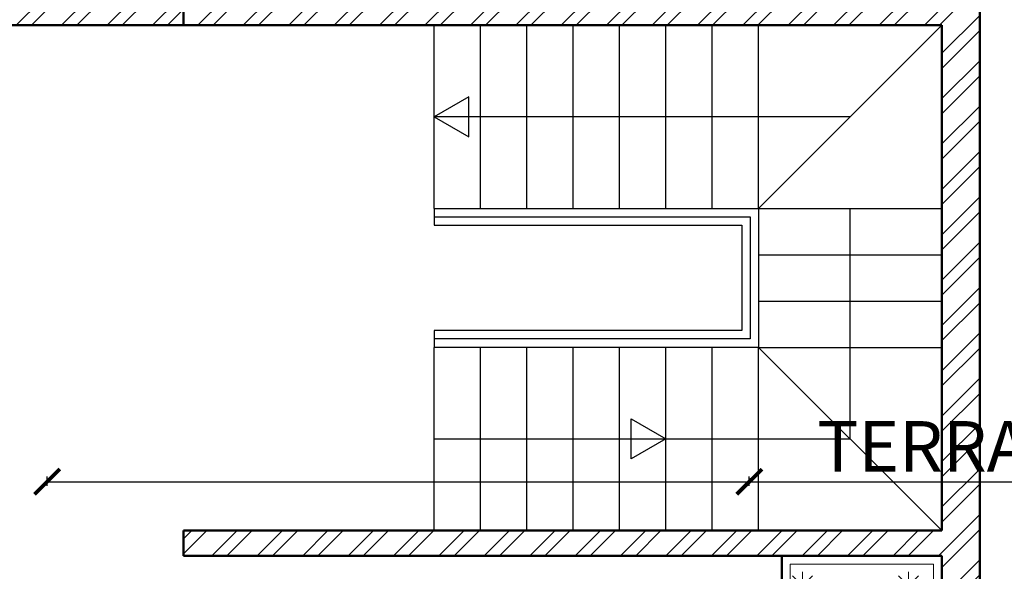
# Model space of a CAD drawing. Units: inches. Extents: x 261 to 2725, y 291 to 1454.
# Tile 32 of 35: x 2266 to 2500, y 670 to 801. Entities that reach past the tile are written whole.
import ezdxf

# ---------------------------------------------------------------- set-up
doc = ezdxf.new("R2010")
doc.units = ezdxf.units.IN
for name, color, linetype, lineweight in [('A-ANNO-DIMS', 136, 'Continuous', 18), ('A-FLOR-STRS', 42, 'Continuous', 25), ('A-PLNT', 3, 'Continuous', 18), ('A-PLNT-PATT', 3, 'Continuous', 13), ('A-WALL', 222, 'Continuous', 50), ('A-WALL-PATT', 243, 'Continuous', 13)]:
    doc.layers.add(name, color=color, linetype=linetype, lineweight=lineweight)
doc.styles.get("Standard").update_dxf_attribs({"font": 'arial.ttf'})
doc.dimstyles.new('ISO-25', dxfattribs={"dimtxt": 12, "dimasz": 6, "dimexe": 1.25, "dimexo": 0.625, "dimtad": 1, "dimdec": 0, "dimlunit": 3, "dimtxsty": 'Standard', "dimblk": 'ARCHTICK', "dimcen": 2.5, "dimadec": 0, "dimazin": 0, "dimtfac": 1, "dimtdec": 0, "dimtmove": 0, "dimatfit": 3, "dimfxl": 1, "dimfxlon": 1, "dimarcsym": 0})

# ---------------------------------------------------------------- blocks, each defined once
blk = doc.blocks.new('_ArchTick')
at = {"color": 0, "linetype": 'ByBlock', "const_width": 0.15}
blk.add_lwpolyline([(-0.5, -0.5), (0.5, 0.5)], dxfattribs=at)
blk = doc.blocks.new('*D71')
at = {"layer": 'A-ANNO-DIMS', "color": 0, "lineweight": -2, "ltscale": 0.07, "transparency": 16777216}
for p, q in [((2272.38, 690.06), (2272.38, 692.31)), ((2439.01, 690.06), (2439.01, 692.31)), ((2272.38, 691.06), (2439.01, 691.06)), ((2439.01, 691.06), (2725.34, 691.06))]:
    blk.add_line(p, q, dxfattribs=at)
at = {"layer": 'Defpoints', "color": 0, "ltscale": 0.07, "transparency": 16777216}
for p in [(2439.01, 691.06), (2272.38, 666.07), (2439.01, 666.07)]:
    blk.add_point(p, dxfattribs=at)
at = {"layer": 'A-ANNO-DIMS', "color": 0, "lineweight": -2, "ltscale": 0.07, "transparency": 16777216, "xscale": 6, "yscale": 6, "zscale": 6, "rotation": 180}
blk.add_blockref('_ArchTick', (2272.38, 691.06), dxfattribs=at)
at = {"layer": 'A-ANNO-DIMS', "color": 0, "lineweight": -2, "ltscale": 0.07, "transparency": 16777216, "xscale": 6, "yscale": 6, "zscale": 6}
blk.add_blockref('_ArchTick', (2439.01, 691.06), dxfattribs=at)
at = {"layer": 'A-ANNO-DIMS', "color": 0, "ltscale": 0.07, "transparency": 16777216, "insert": (2585.18, 697.9), "char_height": 12, "attachment_point": 5}
blk.add_mtext('TERRACE SEATING SET 13\'-10 1/2"', dxfattribs=at)
blk = doc.blocks.new('*D82')
at = {"layer": 'A-ANNO-DIMS', "color": 0, "lineweight": -2, "ltscale": 0.07, "transparency": 16777216}
for p, q in [((2600.96, 679.47), (2603.21, 679.47)), ((2601.96, 517.47), (2601.96, 679.47)), ((2600.96, 517.47), (2603.21, 517.47))]:
    blk.add_line(p, q, dxfattribs=at)
at = {"layer": 'Defpoints', "color": 0, "ltscale": 0.07, "transparency": 16777216}
for p in [(946.45, 679.47), (2601.96, 679.47), (946.45, 517.47)]:
    blk.add_point(p, dxfattribs=at)
at = {"layer": 'A-ANNO-DIMS', "color": 0, "lineweight": -2, "ltscale": 0.07, "transparency": 16777216, "xscale": 6, "yscale": 6, "zscale": 6}
for p, rotation in [((2601.96, 679.47), 90), ((2601.96, 517.47), 270)]:
    blk.add_blockref('_ArchTick', p, dxfattribs=dict(at, rotation=rotation))
at = {"layer": 'A-ANNO-DIMS', "color": 0, "ltscale": 0.07, "transparency": 16777216, "insert": (2595.2, 598.47), "char_height": 12, "attachment_point": 5, "rotation": 90}
blk.add_mtext('13\'-6"', dxfattribs=at)
blk = doc.blocks.new('*D83')
at = {"layer": 'A-ANNO-DIMS', "color": 0, "lineweight": -2, "ltscale": 0.07, "transparency": 16777216}
for p, q in [((2600.96, 799.47), (2603.21, 799.47)), ((2601.96, 679.47), (2601.96, 799.47)), ((2600.96, 679.47), (2603.21, 679.47))]:
    blk.add_line(p, q, dxfattribs=at)
at = {"layer": 'Defpoints', "color": 0, "ltscale": 0.07, "transparency": 16777216}
for p in [(946.45, 799.47), (2601.96, 799.47), (946.45, 679.47)]:
    blk.add_point(p, dxfattribs=at)
at = {"layer": 'A-ANNO-DIMS', "color": 0, "lineweight": -2, "ltscale": 0.07, "transparency": 16777216, "xscale": 6, "yscale": 6, "zscale": 6}
for p, rotation in [((2601.96, 799.47), 90), ((2601.96, 679.47), 270)]:
    blk.add_blockref('_ArchTick', p, dxfattribs=dict(at, rotation=rotation))
at = {"layer": 'A-ANNO-DIMS', "color": 0, "ltscale": 0.07, "transparency": 16777216, "insert": (2595.21, 739.47), "char_height": 12, "attachment_point": 5, "rotation": 90}
blk.add_mtext('10\'-0"', dxfattribs=at)
blk = doc.blocks.new('*D84')
at = {"layer": 'A-ANNO-DIMS', "color": 0, "lineweight": -2, "ltscale": 0.07, "transparency": 16777216}
for p, q in [((2600.96, 1024.47), (2603.21, 1024.47)), ((2601.96, 799.47), (2601.96, 1024.47)), ((2600.96, 799.47), (2603.21, 799.47))]:
    blk.add_line(p, q, dxfattribs=at)
at = {"layer": 'Defpoints', "color": 0, "ltscale": 0.07, "transparency": 16777216}
for p in [(946.45, 1024.47), (2601.96, 1024.47), (946.45, 799.47)]:
    blk.add_point(p, dxfattribs=at)
at = {"layer": 'A-ANNO-DIMS', "color": 0, "lineweight": -2, "ltscale": 0.07, "transparency": 16777216, "xscale": 6, "yscale": 6, "zscale": 6}
for p, rotation in [((2601.96, 1024.47), 90), ((2601.96, 799.47), 270)]:
    blk.add_blockref('_ArchTick', p, dxfattribs=dict(at, rotation=rotation))
at = {"layer": 'A-ANNO-DIMS', "color": 0, "ltscale": 0.07, "transparency": 16777216, "insert": (2595.21, 911.97), "char_height": 12, "attachment_point": 5, "rotation": 90}
blk.add_mtext('18\'-9"', dxfattribs=at)
blk = doc.blocks.new('*D112')
at = {"layer": 'A-ANNO-DIMS', "color": 0, "lineweight": -2, "ltscale": 0.07, "transparency": 16777216}
for p, q in [((2600.96, 679.47), (2603.21, 679.47)), ((2601.96, 550.47), (2601.96, 679.47)), ((2600.96, 550.47), (2603.21, 550.47))]:
    blk.add_line(p, q, dxfattribs=at)
at = {"layer": 'Defpoints', "color": 0, "ltscale": 0.07, "transparency": 16777216}
for p in [(1720.08, 679.47), (2601.96, 679.47), (1720.08, 550.47)]:
    blk.add_point(p, dxfattribs=at)
at = {"layer": 'A-ANNO-DIMS', "color": 0, "lineweight": -2, "ltscale": 0.07, "transparency": 16777216, "xscale": 6, "yscale": 6, "zscale": 6}
for p, rotation in [((2601.96, 679.47), 90), ((2601.96, 550.47), 270)]:
    blk.add_blockref('_ArchTick', p, dxfattribs=dict(at, rotation=rotation))
at = {"layer": 'A-ANNO-DIMS', "color": 0, "ltscale": 0.07, "transparency": 16777216, "insert": (2595.21, 614.97), "char_height": 12, "attachment_point": 5, "rotation": 90}
blk.add_mtext('10\'-9"', dxfattribs=at)
blk = doc.blocks.new('*D113')
at = {"layer": 'A-ANNO-DIMS', "color": 0, "lineweight": -2, "ltscale": 0.07, "transparency": 16777216}
for p, q in [((2600.96, 799.47), (2603.21, 799.47)), ((2601.96, 679.47), (2601.96, 799.47)), ((2600.96, 679.47), (2603.21, 679.47))]:
    blk.add_line(p, q, dxfattribs=at)
at = {"layer": 'Defpoints', "color": 0, "ltscale": 0.07, "transparency": 16777216}
for p in [(1720.08, 799.47), (2601.96, 799.47), (1720.08, 679.47)]:
    blk.add_point(p, dxfattribs=at)
at = {"layer": 'A-ANNO-DIMS', "color": 0, "lineweight": -2, "ltscale": 0.07, "transparency": 16777216, "xscale": 6, "yscale": 6, "zscale": 6}
for p, rotation in [((2601.96, 799.47), 90), ((2601.96, 679.47), 270)]:
    blk.add_blockref('_ArchTick', p, dxfattribs=dict(at, rotation=rotation))
at = {"layer": 'A-ANNO-DIMS', "color": 0, "ltscale": 0.07, "transparency": 16777216, "insert": (2595.21, 739.47), "char_height": 12, "attachment_point": 5, "rotation": 90}
blk.add_mtext('10\'-0"', dxfattribs=at)
blk = doc.blocks.new('*D114')
at = {"layer": 'A-ANNO-DIMS', "color": 0, "lineweight": -2, "ltscale": 0.07, "transparency": 16777216}
for p, q in [((2600.96, 964.47), (2603.21, 964.47)), ((2601.96, 799.47), (2601.96, 964.47)), ((2600.96, 799.47), (2603.21, 799.47))]:
    blk.add_line(p, q, dxfattribs=at)
at = {"layer": 'Defpoints', "color": 0, "ltscale": 0.07, "transparency": 16777216}
for p in [(1720.08, 964.47), (2601.96, 964.47), (1720.08, 799.47)]:
    blk.add_point(p, dxfattribs=at)
at = {"layer": 'A-ANNO-DIMS', "color": 0, "lineweight": -2, "ltscale": 0.07, "transparency": 16777216, "xscale": 6, "yscale": 6, "zscale": 6}
for p, rotation in [((2601.96, 964.47), 90), ((2601.96, 799.47), 270)]:
    blk.add_blockref('_ArchTick', p, dxfattribs=dict(at, rotation=rotation))
at = {"layer": 'A-ANNO-DIMS', "color": 0, "ltscale": 0.07, "transparency": 16777216, "insert": (2595.2, 881.97), "char_height": 12, "attachment_point": 5, "rotation": 90}
blk.add_mtext('13\'-9"', dxfattribs=at)
blk = doc.blocks.new('*D126')
at = {"layer": 'A-ANNO-DIMS', "color": 0, "lineweight": -2, "ltscale": 0.07, "transparency": 16777216}
for p, q in [((2600.96, 673.47), (2603.21, 673.47)), ((2601.96, 496.47), (2601.96, 673.47)), ((2600.96, 496.47), (2603.21, 496.47))]:
    blk.add_line(p, q, dxfattribs=at)
at = {"layer": 'Defpoints', "color": 0, "ltscale": 0.07, "transparency": 16777216}
for p in [(2484.71, 673.47), (2601.96, 673.47), (2493.71, 496.47)]:
    blk.add_point(p, dxfattribs=at)
at = {"layer": 'A-ANNO-DIMS', "color": 0, "lineweight": -2, "ltscale": 0.07, "transparency": 16777216, "xscale": 6, "yscale": 6, "zscale": 6}
for p, rotation in [((2601.96, 673.47), 90), ((2601.96, 496.47), 270)]:
    blk.add_blockref('_ArchTick', p, dxfattribs=dict(at, rotation=rotation))
at = {"layer": 'A-ANNO-DIMS', "color": 0, "ltscale": 0.07, "transparency": 16777216, "insert": (2595.21, 584.97), "char_height": 12, "attachment_point": 5, "rotation": 90}
blk.add_mtext('14\'-9"', dxfattribs=at)
blk = doc.blocks.new('*D127')
at = {"layer": 'A-ANNO-DIMS', "color": 0, "lineweight": -2, "ltscale": 0.07, "transparency": 16777216}
for p, q in [((2600.96, 805.47), (2603.21, 805.47)), ((2601.96, 673.47), (2601.96, 805.47)), ((2600.96, 673.47), (2603.21, 673.47))]:
    blk.add_line(p, q, dxfattribs=at)
at = {"layer": 'Defpoints', "color": 0, "ltscale": 0.07, "transparency": 16777216}
for p in [(2484.71, 805.47), (2601.96, 805.47), (2484.71, 673.47)]:
    blk.add_point(p, dxfattribs=at)
at = {"layer": 'A-ANNO-DIMS', "color": 0, "lineweight": -2, "ltscale": 0.07, "transparency": 16777216, "xscale": 6, "yscale": 6, "zscale": 6}
for p, rotation in [((2601.96, 805.47), 90), ((2601.96, 673.47), 270)]:
    blk.add_blockref('_ArchTick', p, dxfattribs=dict(at, rotation=rotation))
at = {"layer": 'A-ANNO-DIMS', "color": 0, "ltscale": 0.07, "transparency": 16777216, "insert": (2595.21, 739.47), "char_height": 12, "attachment_point": 5, "rotation": 90}
blk.add_mtext('11\'-0"', dxfattribs=at)
blk = doc.blocks.new('*D131')
at = {"layer": 'A-ANNO-DIMS', "color": 0, "lineweight": -2, "ltscale": 0.07, "transparency": 16777216}
for p, q in [((2448.71, 305.22), (2448.71, 302.97)), ((2448.71, 304.22), (2484.71, 304.22)), ((2484.71, 305.22), (2484.71, 302.97))]:
    blk.add_line(p, q, dxfattribs=at)
at = {"layer": 'Defpoints', "color": 0, "ltscale": 0.07, "transparency": 16777216}
for p in [(2484.71, 673.47), (2448.71, 671.47), (2484.71, 304.22)]:
    blk.add_point(p, dxfattribs=at)
at = {"layer": 'A-ANNO-DIMS', "color": 0, "lineweight": -2, "ltscale": 0.07, "transparency": 16777216, "xscale": 6, "yscale": 6, "zscale": 6, "rotation": 180}
blk.add_blockref('_ArchTick', (2448.71, 304.22), dxfattribs=at)
at = {"layer": 'A-ANNO-DIMS', "color": 0, "lineweight": -2, "ltscale": 0.07, "transparency": 16777216, "xscale": 6, "yscale": 6, "zscale": 6}
blk.add_blockref('_ArchTick', (2484.71, 304.22), dxfattribs=at)
at = {"layer": 'A-ANNO-DIMS', "color": 0, "ltscale": 0.07, "transparency": 16777216, "insert": (2466.71, 310.97), "char_height": 12, "attachment_point": 5}
blk.add_mtext('3\'-0"', dxfattribs=at)
blk = doc.blocks.new('*D132')
at = {"layer": 'A-ANNO-DIMS', "color": 0, "lineweight": -2, "ltscale": 0.07, "transparency": 16777216}
for p, q in [((2364.21, 305.22), (2364.21, 302.97)), ((2364.21, 304.22), (2484.71, 304.22)), ((2484.71, 305.22), (2484.71, 302.97))]:
    blk.add_line(p, q, dxfattribs=at)
at = {"layer": 'Defpoints', "color": 0, "ltscale": 0.07, "transparency": 16777216}
for p in [(2364.21, 799.47), (2484.71, 799.47), (2484.71, 304.22)]:
    blk.add_point(p, dxfattribs=at)
at = {"layer": 'A-ANNO-DIMS', "color": 0, "lineweight": -2, "ltscale": 0.07, "transparency": 16777216, "xscale": 6, "yscale": 6, "zscale": 6, "rotation": 180}
blk.add_blockref('_ArchTick', (2364.21, 304.22), dxfattribs=at)
at = {"layer": 'A-ANNO-DIMS', "color": 0, "lineweight": -2, "ltscale": 0.07, "transparency": 16777216, "xscale": 6, "yscale": 6, "zscale": 6}
blk.add_blockref('_ArchTick', (2484.71, 304.22), dxfattribs=at)
at = {"layer": 'A-ANNO-DIMS', "color": 0, "ltscale": 0.07, "transparency": 16777216, "insert": (2424.46, 311.05), "char_height": 12, "attachment_point": 5}
blk.add_mtext('10\'-0 1/2"', dxfattribs=at)
blk = doc.blocks.new('*D136')
at = {"layer": 'A-ANNO-DIMS', "color": 0, "lineweight": -2, "ltscale": 0.07, "transparency": 16777216}
for p, q in [((2600.96, 675.78), (2603.21, 675.78)), ((2601.96, 675.78), (2601.96, 475.47)), ((2600.96, 475.47), (2603.21, 475.47))]:
    blk.add_line(p, q, dxfattribs=at)
at = {"layer": 'Defpoints', "color": 0, "ltscale": 0.07, "transparency": 16777216}
for p in [(2208.67, 675.78), (2208.67, 475.47), (2601.96, 475.47)]:
    blk.add_point(p, dxfattribs=at)
at = {"layer": 'A-ANNO-DIMS', "color": 0, "lineweight": -2, "ltscale": 0.07, "transparency": 16777216, "xscale": 6, "yscale": 6, "zscale": 6}
for p, rotation in [((2601.96, 675.78), 90), ((2601.96, 475.47), 270)]:
    blk.add_blockref('_ArchTick', p, dxfattribs=dict(at, rotation=rotation))
at = {"layer": 'A-ANNO-DIMS', "color": 0, "ltscale": 0.07, "transparency": 16777216, "insert": (2595.13, 575.62), "char_height": 12, "attachment_point": 5, "rotation": 90}
blk.add_mtext('16\'-8 1/2"', dxfattribs=at)

msp = doc.modelspace()

# ---------------------------------------------------------------- hatches: boundary and pattern name
at = {"layer": 'A-PLNT-PATT'}
h = msp.add_hatch(dxfattribs=at)
h.set_pattern_fill('GRASS', color=256, scale=0.7)
h.paths.add_polyline_path([(2052.71, 797.47), (2018.71, 797.47), (2018.71, 450.47), (2206.67, 450.47), (2206.67, 507.47), (2482.71, 507.47), (2482.71, 671.47), (2448.71, 671.47), (2448.71, 541.47), (2172.67, 541.47), (2172.67, 484.47), (2052.71, 484.47)])
at = {"layer": 'A-WALL-PATT'}
h = msp.add_hatch(dxfattribs=at)
h.set_pattern_fill('ANSI32', color=256, scale=0.8)
h.paths.add_polyline_path([(478.45, 685.47), (580.45, 685.47), (580.45, 691.47), (577.45, 691.47), (577.45, 694.47), (571.45, 694.47), (571.45, 691.47), (478.45, 691.47), (478.45, 721.47), (469.45, 721.47), (469.45, 508.47), (538.45, 508.47), (538.45, 517.47), (478.45, 517.47)])
h.paths.add_polyline_path([(694.45, 517.47), (676.45, 517.47), (676.45, 646.47), (670.45, 646.47), (670.45, 517.47), (610.45, 517.47), (610.45, 508.47), (694.45, 508.47)])
h.paths.add_polyline_path([(676.45, 784.47), (478.45, 784.47), (478.45, 844.47), (469.45, 844.47), (469.45, 745.47), (478.45, 745.47), (478.45, 775.47), (571.45, 775.47), (571.45, 724.47), (577.45, 724.47), (577.45, 775.47), (670.45, 775.47), (670.45, 691.47), (610.45, 691.47), (610.45, 685.47), (670.45, 685.47), (670.45, 682.47), (676.45, 682.47)])
h.paths.add_polyline_path([(955.45, 880.47), (946.45, 880.47), (946.45, 808.47), (778.45, 808.47), (778.45, 799.47), (946.45, 799.47), (946.45, 517.47), (898.45, 517.47), (898.45, 508.47), (955.45, 508.47)])
h.paths.add_polyline_path([(778.45, 598.47), (772.45, 598.47), (772.45, 517.47), (754.45, 517.47), (754.45, 508.47), (826.45, 508.47), (826.45, 517.47), (778.45, 517.47)])
h.paths.add_polyline_path([(955.45, 1090.47), (946.45, 1090.47), (946.45, 1030.47), (817.45, 1030.47), (817.45, 1024.47), (946.45, 1024.47), (946.45, 952.47), (955.45, 952.47)])
h.paths.add_polyline_path([(955.45, 1231.47), (730.45, 1231.47), (730.45, 1222.47), (772.45, 1222.47), (772.45, 1096.47), (766.45, 1096.47), (766.45, 1090.47), (772.45, 1090.47), (772.45, 1006.47), (712.45, 1006.47), (712.45, 1000.47), (778.45, 1000.47), (778.45, 1024.47), (781.45, 1024.47), (781.45, 1030.47), (778.45, 1030.47), (778.45, 1222.47), (946.45, 1222.47), (946.45, 1162.47), (955.45, 1162.47)])
h.paths.add_polyline_path([(694.45, 1231.47), (619.45, 1231.47), (619.45, 1222.47), (646.45, 1222.47), (646.45, 1039.47), (652.45, 1039.47), (652.45, 1090.47), (736.45, 1090.47), (736.45, 1096.47), (652.45, 1096.47), (652.45, 1222.47), (694.45, 1222.47)])
h.paths.add_polyline_path([(571.45, 1231.47), (469.45, 1231.47), (469.45, 1099.47), (478.45, 1099.47), (478.45, 1144.47), (544.45, 1144.47), (544.45, 1153.47), (538.45, 1153.47), (538.45, 1150.47), (478.45, 1150.47), (478.45, 1222.47), (538.45, 1222.47), (538.45, 1183.47), (544.45, 1183.47), (544.45, 1222.47), (571.45, 1222.47)])
h.paths.add_polyline_path([(538.45, 1006.47), (478.45, 1006.47), (478.45, 1051.47), (469.45, 1051.47), (469.45, 940.47), (478.45, 940.47), (478.45, 1000.47), (538.45, 1000.47)])
h.paths.add_polyline_path([(652.45, 1006.47), (652.45, 1009.47), (646.45, 1009.47), (646.45, 1006.47), (586.45, 1006.47), (586.45, 1000.47), (652.45, 1000.47)])
h.paths.add_polyline_path([(1288.08, 973.47), (1243.08, 973.47), (1243.08, 920.97), (1252.08, 920.97), (1252.08, 964.47), (1288.08, 964.47)], flags=17)
h.paths.add_polyline_path([(1402.08, 805.47), (1252.08, 805.47), (1252.08, 848.97), (1243.08, 848.97), (1243.08, 757.47), (1252.08, 757.47), (1252.08, 799.47), (1294.08, 799.47), (1372.08, 799.47), (1372.08, 779.47), (1372.08, 715.47), (1378.08, 715.47), (1378.08, 799.47), (1402.08, 799.47)])
h.paths.add_polyline_path([(1252.08, 721.47), (1243.08, 721.47), (1243.08, 439.47), (1729.08, 439.47), (1729.08, 709.47), (1720.08, 709.47), (1720.08, 679.47), (1582.08, 679.47), (1582.08, 670.47), (1588.08, 670.47), (1588.08, 673.47), (1720.08, 673.47), (1720.08, 559.47), (1690.08, 559.47), (1690.08, 550.47), (1720.08, 550.47), (1720.08, 448.47), (1252.08, 448.47), (1252.08, 496.47), (1312.08, 496.47), (1312.08, 505.47), (1252.08, 505.47), (1252.08, 673.47), (1405.08, 673.47), (1405.08, 679.47), (1378.08, 679.47), (1378.08, 685.47), (1372.08, 685.47), (1372.08, 679.47), (1252.08, 679.47)])
h.paths.add_polyline_path([(1450.08, 550.47), (1480.08, 550.47), (1480.08, 559.47), (1450.08, 559.47), (1450.08, 679.47), (1441.08, 679.47), (1441.08, 673.47), (1444.08, 673.47), (1444.08, 505.47), (1384.08, 505.47), (1384.08, 496.47), (1450.08, 496.47)], flags=17)
h.paths.add_polyline_path([(1618.08, 559.47), (1588.08, 559.47), (1588.08, 634.47), (1582.08, 634.47), (1582.08, 559.47), (1552.08, 559.47), (1552.08, 550.47), (1618.08, 550.47)], flags=17)
h.paths.add_polyline_path([(1564.08, 964.47), (1630.08, 964.47), (1630.08, 973.47), (1477.08, 973.47), (1477.08, 964.47), (1558.08, 964.47), (1558.08, 926.22), (1558.08, 887.97), (1486.08, 887.97), (1486.08, 881.97), (1558.08, 881.97), (1558.08, 805.47), (1450.08, 805.47), (1450.08, 845.97), (1444.08, 845.97), (1444.08, 805.47), (1438.08, 805.47), (1438.08, 799.47), (1564.08, 799.47)], flags=17)
h.paths.add_polyline_path([(1453.08, 973.47), (1408.08, 973.47), (1408.08, 964.47), (1444.08, 964.47), (1444.08, 881.97), (1450.08, 881.97), (1456.08, 881.97), (1456.08, 887.97), (1450.08, 887.97), (1450.08, 964.47), (1453.08, 964.47)], flags=17)
h.paths.add_polyline_path([(1729.08, 1231.47), (1243.08, 1231.47), (1243.08, 1167.47), (1252.08, 1167.47), (1252.08, 1222.47), (1441.08, 1222.47), (1441.08, 1045.47), (1648.08, 1045.47), (1648.08, 1051.47), (1450.08, 1051.47), (1450.08, 1074.47), (1450.08, 1222.47), (1472.08, 1222.47), (1720.08, 1222.47), (1720.08, 1051.47), (1708.08, 1051.47), (1708.08, 1045.47), (1720.08, 1045.47), (1720.08, 973.47), (1702.08, 973.47), (1702.08, 964.47), (1720.08, 964.47), (1720.08, 769.47), (1729.08, 769.47)])
h.paths.add_polyline_path([(2493.71, 1054.85), (2007.71, 1054.85), (2007.71, 439.47), (2214.67, 439.47), (2214.67, 496.47), (2493.71, 496.47)])
h.paths.add_polyline_path([(2016.71, 1045.85), (2304.71, 1045.85), (2304.71, 841.47), (2310.71, 841.47), (2310.71, 1045.85), (2484.71, 1045.85), (2484.71, 805.47), (2310.71, 805.47), (2310.71, 811.47), (2304.71, 811.47), (2304.71, 799.47), (2484.71, 799.47), (2484.71, 679.47), (2304.71, 679.47), (2304.71, 673.47), (2484.71, 673.47), (2484.71, 505.47), (2208.67, 505.47), (2208.67, 448.47), (2016.71, 448.47), (2016.71, 799.47), (2304.71, 799.47), (2304.71, 805.47), (2016.71, 805.47)], flags=16)

# ---------------------------------------------------------------- linework, layer by layer
at = {"layer": 'A-FLOR-STRS'}
for p, q in [((2364.21, 799.47), (2484.71, 799.47)), ((2364.21, 755.97), (2364.21, 799.47)), ((2375.21, 755.97), (2375.21, 799.47)), ((2386.21, 755.97), (2386.21, 799.47)), ((2397.21, 755.97), (2397.21, 799.47)), ((2408.21, 755.97), (2408.21, 799.47)), ((2419.21, 755.97), (2419.21, 799.47)), ((2430.21, 755.97), (2430.21, 799.47)), ((2441.21, 755.97), (2441.21, 799.47)), ((2441.21, 755.97), (2484.71, 799.47)), ((2484.71, 679.47), (2484.71, 799.47)), ((2462.96, 777.72), (2364.21, 777.72)), ((2364.21, 755.97), (2364.21, 751.97)), ((2441.21, 755.97), (2484.71, 755.97)), ((2462.96, 701.22), (2462.96, 755.97)), ((2441.21, 744.97), (2484.71, 744.97)), ((2441.21, 733.97), (2484.71, 733.97)), ((2364.21, 726.97), (2364.21, 722.97)), ((2364.21, 679.47), (2364.21, 722.97)), ((2375.21, 679.47), (2375.21, 722.97)), ((2386.21, 679.47), (2386.21, 722.97)), ((2397.21, 679.47), (2397.21, 722.97)), ((2408.21, 679.47), (2408.21, 722.97)), ((2419.21, 679.47), (2419.21, 722.97)), ((2430.21, 679.47), (2430.21, 722.97)), ((2441.21, 722.97), (2484.71, 722.97)), ((2441.21, 679.47), (2441.21, 722.97)), ((2441.21, 722.97), (2484.71, 679.47)), ((2364.21, 701.22), (2462.96, 701.22)), ((2364.21, 679.47), (2484.71, 679.47))]:
    msp.add_line(p, q, dxfattribs=at)
for points in [[(2364.21, 777.72), (2372.46, 772.96), (2372.46, 782.48)], [(2419.21, 701.22), (2410.96, 696.46), (2410.96, 705.98)]]:
    msp.add_lwpolyline(points, close=True, dxfattribs=at)
for points in [[(2364.21, 755.97), (2441.21, 755.97), (2441.21, 722.97), (2364.21, 722.97)], [(2364.21, 753.97), (2439.21, 753.97), (2439.21, 724.97), (2364.21, 724.97)], [(2364.21, 751.97), (2437.21, 751.97), (2437.21, 726.97), (2364.21, 726.97)]]:
    msp.add_lwpolyline(points, dxfattribs=at)
at = {"layer": 'A-PLNT'}
msp.add_line((2482.71, 671.47), (2448.71, 671.47), dxfattribs=at)
for points in [[(2018.71, 797.47), (2018.71, 450.47), (2206.67, 450.47), (2206.67, 507.47), (2482.71, 507.47), (2482.71, 671.47)], [(2052.71, 797.47), (2052.71, 484.47), (2172.67, 484.47), (2172.67, 541.47), (2448.71, 541.47), (2448.71, 671.47)]]:
    msp.add_lwpolyline(points, dxfattribs=at)
at = {"layer": 'A-WALL'}
for p, q in [((2493.71, 1054.85), (2493.71, 496.47)), ((2304.71, 811.47), (2304.71, 799.47)), ((2016.71, 799.47), (2484.71, 799.47)), ((2484.71, 799.47), (2484.71, 679.47)), ((2304.71, 679.47), (2484.71, 679.47)), ((2304.71, 679.47), (2304.71, 673.47)), ((2304.71, 673.47), (2484.71, 673.47))]:
    msp.add_line(p, q, dxfattribs=at)
for points in [[(2016.71, 799.47), (2016.71, 448.47), (2208.67, 448.47), (2208.67, 505.47), (2484.71, 505.47), (2484.71, 673.47)], [(2054.71, 799.47), (2054.71, 486.47), (2170.67, 486.47), (2170.67, 543.47), (2446.71, 543.47), (2446.71, 673.47)]]:
    msp.add_lwpolyline(points, dxfattribs=at)

# ---------------------------------------------------------------- dimensions: what is measured, and where the dimension line sits
at = {"layer": 'A-ANNO-DIMS', "ltscale": 0.07}
for base, p1, p2, picture, middle in [((2601.96, 1024.47), (946.45, 799.47), (946.45, 1024.47), '*D84', (2595.21, 911.97)), ((2601.96, 964.47), (1720.08, 799.47), (1720.08, 964.47), '*D114', (2595.2, 881.97)), ((2601.96, 805.47), (2484.71, 673.47), (2484.71, 805.47), '*D127', (2595.21, 739.47)), ((2601.96, 799.47), (946.45, 679.47), (946.45, 799.47), '*D83', (2595.21, 739.47)), ((2601.96, 799.47), (1720.08, 679.47), (1720.08, 799.47), '*D113', (2595.21, 739.47)), ((2601.96, 679.47), (946.45, 517.47), (946.45, 679.47), '*D82', (2595.2, 598.47)), ((2601.96, 679.47), (1720.08, 550.47), (1720.08, 679.47), '*D112', (2595.21, 614.97)), ((2601.96, 475.47), (2208.67, 675.78), (2208.67, 475.47), '*D136', (2595.13, 575.62)), ((2601.96, 673.47), (2493.71, 496.47), (2484.71, 673.47), '*D126', (2595.21, 584.97))]:
    dim = msp.add_linear_dim(base=base, p1=p1, p2=p2, angle=90, dimstyle='ISO-25', override={"dimdec": 1, "dimlfac": 1, "dimrnd": 0, "dimzin": 1, "dimdsep": 46, "dimlunit": 4, "dimfrac": 2}, dxfattribs=at)
    dim.commit()
    dim.dimension.update_dxf_attribs({"geometry": picture, "text_midpoint": middle})
for p1, p2, picture, middle in [((2364.21, 799.47), (2484.71, 799.47), '*D132', (2424.46, 311.05)), ((2448.71, 671.47), (2484.71, 673.47), '*D131', (2466.71, 310.97))]:
    dim = msp.add_linear_dim(base=(2484.71, 304.22), p1=p1, p2=p2, dimstyle='ISO-25', override={"dimdec": 1, "dimlfac": 1, "dimrnd": 0, "dimzin": 1, "dimdsep": 46, "dimlunit": 4, "dimfrac": 2}, dxfattribs=at)
    dim.commit()
    dim.dimension.update_dxf_attribs({"geometry": picture, "text_midpoint": middle})
dim = msp.add_linear_dim(base=(2439.01, 691.06), p1=(2272.38, 666.07), p2=(2439.01, 666.07), text='TERRACE SEATING SET <>', dimstyle='ISO-25', override={"dimdec": 1, "dimrnd": 0, "dimzin": 1, "dimlunit": 4, "dimfrac": 2}, dxfattribs=at)
dim.commit()
dim.dimension.update_dxf_attribs({"geometry": '*D71', "text_midpoint": (2585.18, 697.9)})

doc.saveas('drawing.dxf')
